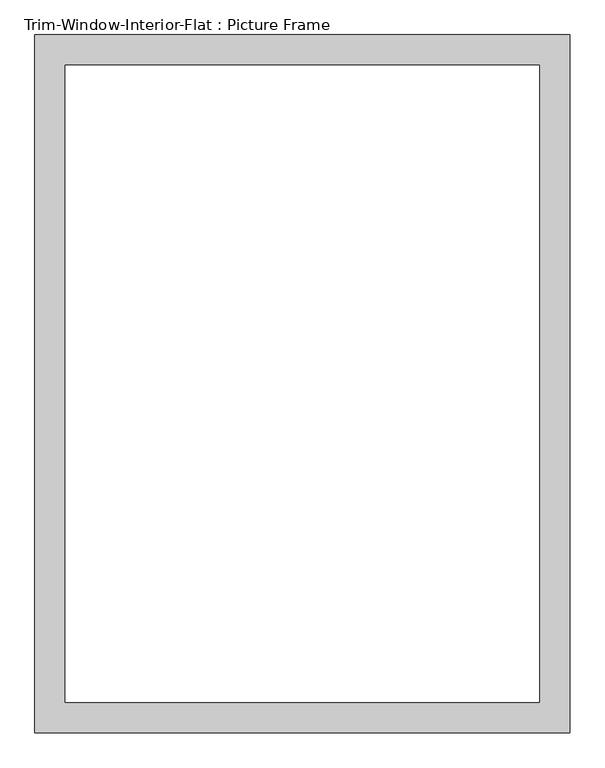
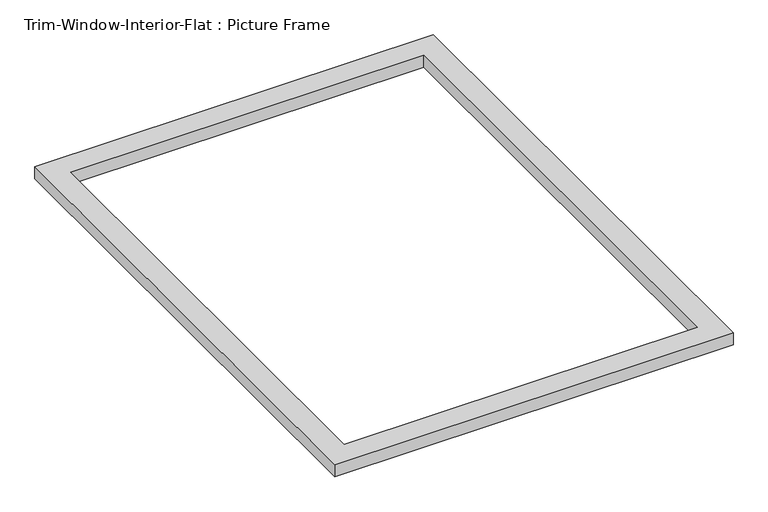
"""IFC4 building model written with IfcOpenShell, lengths in millimetres: proxy geometry, Trim-Window-Interior-Flat : Picture Frame."""

from ifc_helpers import new_model, si_unit, origin, origin_with_axes, place, context, project, spatial, polyline, outline, extrude, source, transform, mapped, element, save


def trim_window_interior_flat_picture_frame_39ff4276(model_context):
    return source(origin(), model_context, "Body", "SweptSolid", [
        extrude(outline(polyline([(501.65, 44.45), (501.65, -1263.65), (-501.65, -1263.65), (-501.65, 44.45), (501.65, 44.45)]), holes=[polyline([(444.5, -12.7), (-444.5, -12.7), (-444.5, -1206.5), (444.5, -1206.5), (444.5, -12.7)])]), origin_with_axes(), (0.0, 0.0, 1.0), 31.75),
    ])


if __name__ == "__main__":
    model = new_model("IFC4")
    model_context = context("Model", 3, world=origin())
    ifc_project = project(units=[si_unit("LENGTHUNIT", "METRE", prefix="MILLI")], contexts=[model_context])
    site = spatial("IfcSite", under=ifc_project)
    building = spatial("IfcBuilding", under=site)
    placement = place(None, origin())
    trim_window_interior_flat_picture_frame_shape = trim_window_interior_flat_picture_frame_39ff4276(model_context)
    element("IfcBuildingElementProxy", 1, Name="Trim-Window-Interior-Flat : Picture Frame", ObjectType="Trim-Window-Interior-Flat : Picture Frame", at=placement, inside=building, context=model_context, shape_type="MappedRepresentation", body=[
        mapped(trim_window_interior_flat_picture_frame_shape, transform((0.0, 0.0, 0.0), x_axis=(1.0, 0.0, 0.0), y_axis=(0.0, 1.0, 0.0), z_axis=(0.0, 0.0, 1.0))),
    ])
    save(model, "model.ifc")

# Revit data of these elements
# Type "Trim-Window-Interior-Flat : Picture Frame"
#   Trim Thickness_Picture Frame = 0' - 1 1/4"
#   Trim Width = 0' - 2 1/4"
#   Trim Thickness_with Sill = 0' - 0 3/4"
#   Sill Thickness = 0' - 1 1/4"
#   Opening Width [instance default] = 2' - 0"
#   Opening Height [instance default] = 3' - 0"
#   Default Elevation = 4' - 0"
#   Sill = no
#   Picture Frame = yes
#   Trim Material [instance default] = none
# Element 1 (IfcBuildingElementProxy, "Trim-Window-Interior-Flat : Picture Frame")
#   Opening Width = 3' - 0"
#   Opening Height = 4' - 0"
#   Trim Material = Wood - Stained
#   Materials on its faces: "Wood - Stained"
# Materials
#   "Wood - Stained": class "Wood", colour RGB 173 132 96, transparency 0, Cost = 0
